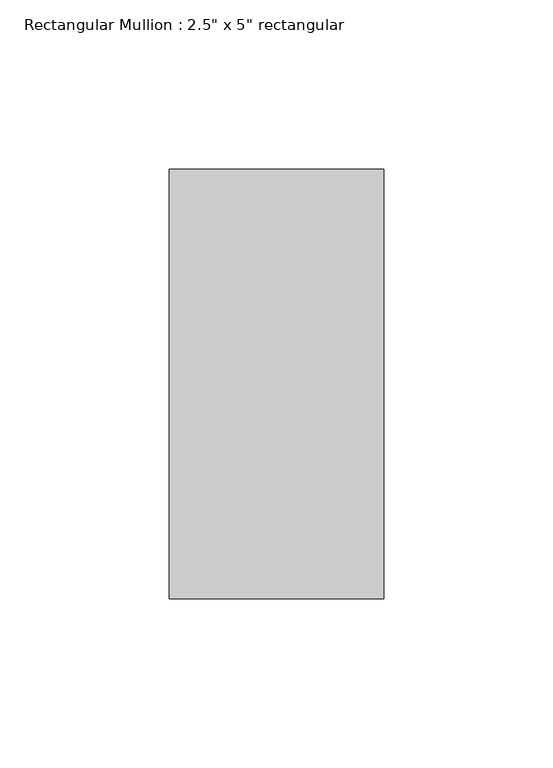
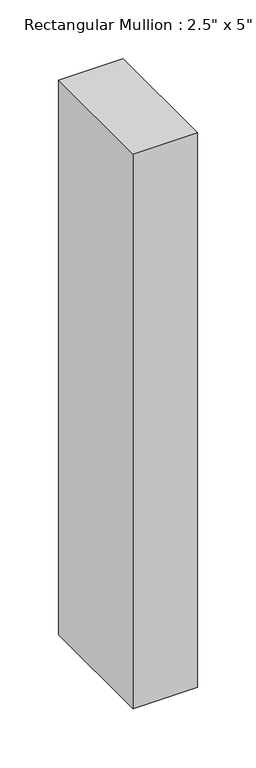
"""IFC4 building model written with IfcOpenShell, lengths in millimetres: member geometry."""

from ifc_helpers import new_model, si_unit, frame, origin, place, context, project, spatial, polyline, outline, extrude, source, transform, mapped, element, save


def member_830eb86c(model_context):
    return source(origin(), model_context, "Body", "SweptSolid", [
        extrude(outline(polyline([(0.0, 63.5), (0.0, -63.5), (-63.5, -63.5), (-63.5, 63.5), (0.0, 63.5)])), frame((0.0, 0.0, -577.85), z_axis=(0.0, 0.0, 1.0), x_axis=(1.0, 0.0, 0.0)), (0.0, 0.0, 1.0), 577.85),
    ])


if __name__ == "__main__":
    model = new_model("IFC4")
    model_context = context("Model", 3, world=origin())
    ifc_project = project(units=[si_unit("LENGTHUNIT", "METRE", prefix="MILLI")], contexts=[model_context])
    site = spatial("IfcSite", under=ifc_project)
    building = spatial("IfcBuilding", under=site)
    placement = place(None, origin())
    member_shape = member_830eb86c(model_context)
    element("IfcMember", 1, ObjectType="Rectangular Mullion : 2.5\" x 5\" rectangular", at=placement, inside=building, context=model_context, shape_type="MappedRepresentation", body=[
        mapped(member_shape, transform((0.0, 0.0, 0.0), x_axis=(1.0, 0.0, 0.0), y_axis=(0.0, 1.0, 0.0), z_axis=(0.0, 0.0, 1.0))),
    ])
    save(model, "model.ifc")

# Revit data of these elements
# Type "Rectangular Mullion : 2.5\" x 5\" rectangular"
#   built-in parameter 1007304 = 0.416667 (stored number, unit not read)
#   built-in parameter 1007301 = 0.104167 (stored number, unit not read)
#   built-in parameter 1007300 = 0.104167 (stored number, unit not read)
# Element 1 (IfcMember, "Rectangular Mullion : 2.5\" x 5\" rectangular")
#   Materials on its faces: "Aluminum"
# Materials
#   "Aluminum": class "Metal", colour RGB 247 247 247, transparency 0, Description = "Aluminum 6061", Cost = 0
